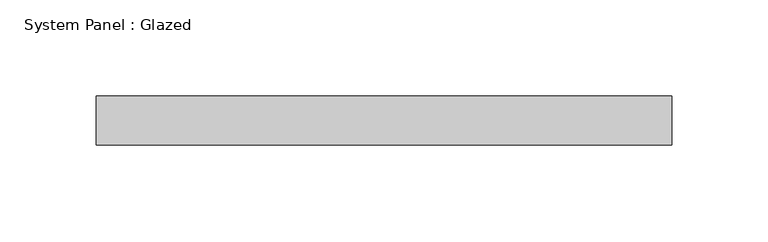
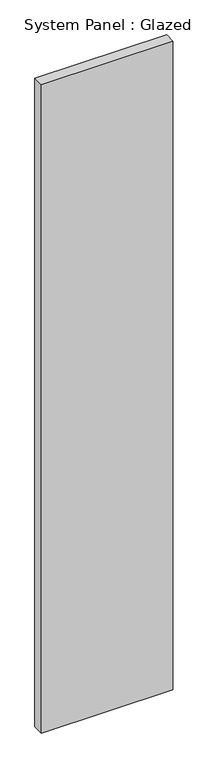
"""IFC4 building model written with IfcOpenShell, lengths in millimetres: plate geometry, System Panel : Glazed."""

from ifc_helpers import new_model, si_unit, origin, origin_with_axes, place, context, project, spatial, polyline, outline, extrude, source, transform, mapped, element, save


def system_panel_glazed_93f5a346(model_context):
    return source(origin(), model_context, "Body", "SweptSolid", [
        extrude(outline(polyline([(149.225, 19.05), (-149.225, 19.05), (-149.225, 44.45), (149.225, 44.45), (149.225, 19.05)])), origin_with_axes(), (0.0, 0.0, 1.0), 1554.1349385),
    ])


if __name__ == "__main__":
    model = new_model("IFC4")
    model_context = context("Model", 3, world=origin())
    ifc_project = project(units=[si_unit("LENGTHUNIT", "METRE", prefix="MILLI")], contexts=[model_context])
    site = spatial("IfcSite", under=ifc_project)
    building = spatial("IfcBuilding", under=site)
    placement = place(None, origin())
    system_panel_glazed_shape = system_panel_glazed_93f5a346(model_context)
    element("IfcPlate", 1, ObjectType="System Panel : Glazed", at=placement, inside=building, context=model_context, shape_type="MappedRepresentation", body=[
        mapped(system_panel_glazed_shape, transform((0.0, 0.0, 0.0), x_axis=(1.0, 0.0, 0.0), y_axis=(0.0, 1.0, 0.0), z_axis=(0.0, 0.0, 1.0))),
    ])
    save(model, "model.ifc")

# Revit data of these elements
# Type "System Panel : Glazed"
#   Construction Type Id = "GSP4R"
#   Analytic Construction = "1/8 in Pilkington single glazing"
#   Visual Light Transmittance = 0.9
#   Solar Heat Gain Coefficient = 0.86
#   Heat Transfer Coefficient (U) = 1.18115 BTU/(h·ft²·°F)
#   Define Thermal Properties by = 1
# Element 1 (IfcPlate, "System Panel : Glazed")
#   Materials on its faces: "Glass"
# Materials
#   "Glass": class "Glass", colour RGB 0 128 192, transparency 0.75, Description = "Soda Lime Glass", Cost = 0
